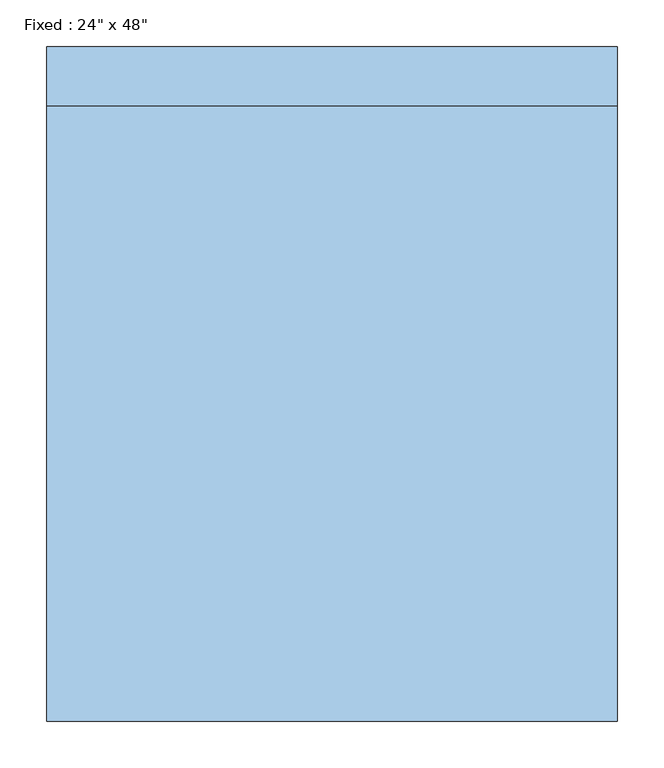
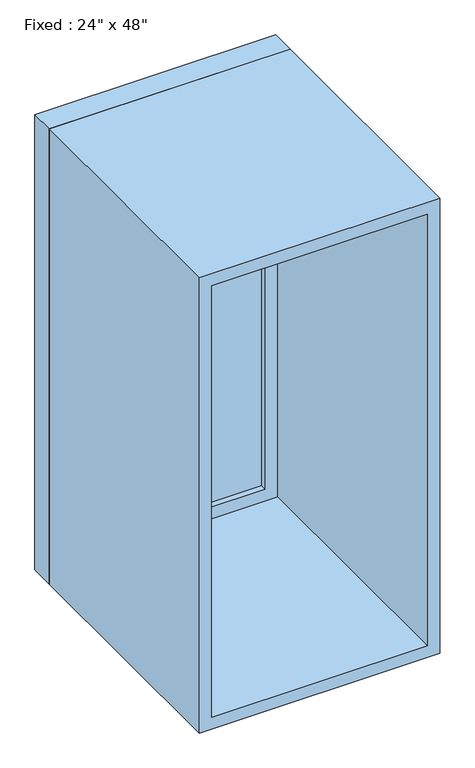
"""IFC4 building model written with IfcOpenShell, lengths in millimetres: window geometry."""

from ifc_helpers import new_model, si_unit, frame, origin, place, context, project, spatial, polyline, outline, extrude, source, transform, mapped, element, save


def window_df4b05bc(model_context):
    return source(origin(), model_context, "Body", "SweptSolid", [
        extrude(outline(polyline([(203.2, 312.7209496), (-279.4, 312.7209496), (-279.4, 325.4209496), (203.2, 325.4209496), (203.2, 312.7209496)])), frame((0.0, 0.0, 977.9), z_axis=(0.0, 0.0, 1.0), x_axis=(1.0, 0.0, 0.0)), (0.0, 0.0, 1.0), 1092.2),
        extrude(outline(polyline([(2114.55, -323.85), (933.45, -323.85), (933.45, 247.65), (2114.55, 247.65), (2114.55, -323.85)]), holes=[polyline([(2070.1, -279.4), (2070.1, 203.2), (977.9, 203.2), (977.9, -279.4), (2070.1, -279.4)])]), frame((0.0, 296.8459496, 0.0), z_axis=(0.0, 1.0, 0.0), x_axis=(0.0, 0.0, 1.0)), (0.0, 0.0, 1.0), 44.45),
        extrude(outline(polyline([(2133.6, -342.9), (914.4, -342.9), (914.4, 266.7), (2133.6, 266.7), (2133.6, -342.9)]), holes=[polyline([(2101.85, -311.15), (2101.85, 234.95), (946.15, 234.95), (946.15, -311.15), (2101.85, -311.15)])]), frame((0.0, -360.3459496, 0.0), z_axis=(0.0, 1.0, 0.0), x_axis=(0.0, 0.0, 1.0)), (0.0, 0.0, 1.0), 657.1918992),
        extrude(outline(polyline([(2133.6, 266.7), (2133.6, -342.9), (914.4, -342.9), (914.4, 266.7), (2133.6, 266.7)]), holes=[polyline([(2114.55, 247.65), (933.45, 247.65), (933.45, -323.85), (2114.55, -323.85), (2114.55, 247.65)])]), frame((0.0, 296.8459496, 0.0), z_axis=(0.0, 1.0, 0.0), x_axis=(0.0, 0.0, 1.0)), (0.0, 0.0, 1.0), 63.5),
    ])


if __name__ == "__main__":
    model = new_model("IFC4")
    model_context = context("Model", 3, world=origin())
    ifc_project = project(units=[si_unit("LENGTHUNIT", "METRE", prefix="MILLI")], contexts=[model_context])
    site = spatial("IfcSite", under=ifc_project)
    building = spatial("IfcBuilding", under=site)
    placement = place(None, origin())
    window_shape = window_df4b05bc(model_context)
    element("IfcWindow", 1, ObjectType="Fixed : 24\" x 48\"", at=placement, inside=building, context=model_context, shape_type="MappedRepresentation", body=[
        mapped(window_shape, transform((0.0, 0.0, 0.0), x_axis=(1.0, 0.0, 0.0), y_axis=(0.0, 1.0, 0.0), z_axis=(0.0, 0.0, 1.0))),
    ])
    save(model, "model.ifc")

# Revit data of these elements
# Type "Fixed : 24\" x 48\""
#   Type Mark = "2"
#   Construction Type Id = "GSP4R"
#   Assembly Code = "B2020100"
#   Analytic Construction = "1/8 in Pilkington single glazing"
#   Visual Light Transmittance = 0.9
#   Solar Heat Gain Coefficient = 0.78
#   Heat Transfer Coefficient (U) = 0.6496 BTU/(h·ft²·°F)
#   Height = 4' - 0"
#   Default Sill Height = 3' - 0"
#   Width = 2' - 0"
#   Window Inset = 0' - 0 3/4"
#   Define Thermal Properties by = 1
#   Glass Pane Material = Glass
#   Sash Material = Sash
#   Wall Closure = (empty or 0)
# Element 1 (IfcWindow, "Fixed : 24\" x 48\"")
#   Materials on its faces: "Sash", "Glass"
# Materials
#   "Glass": class "Glass", colour RGB 0 128 192, transparency 0.75, Description = "Soda Lime Glass", Cost = 0
#   "Sash": class "Wood", colour RGB 224 178 126, transparency 0
